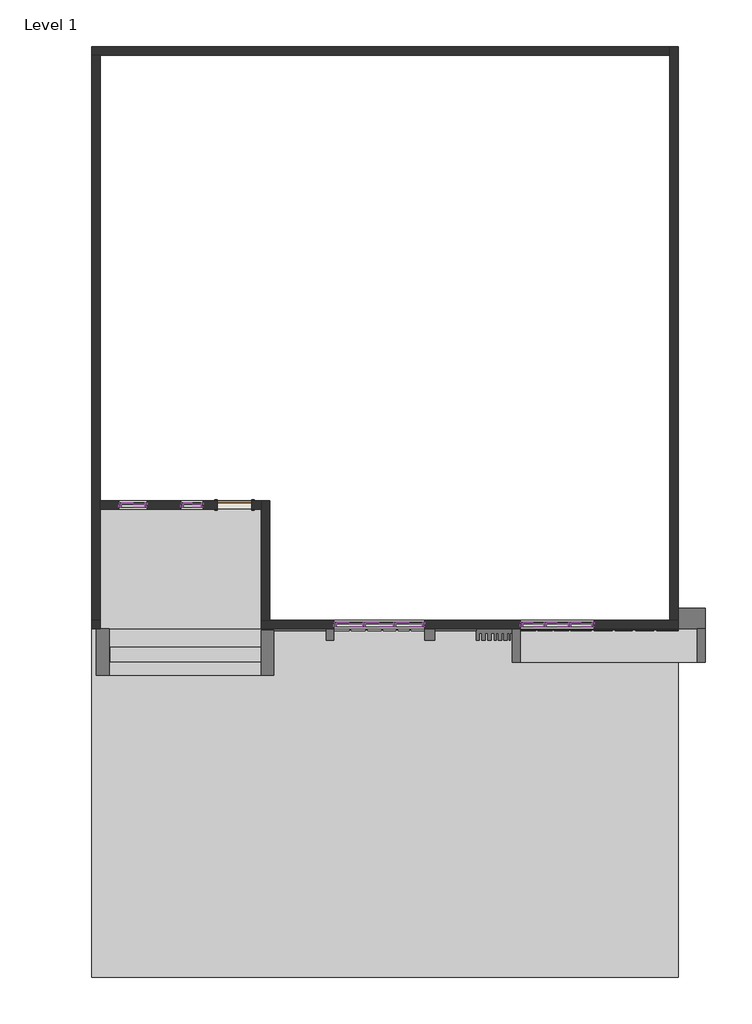
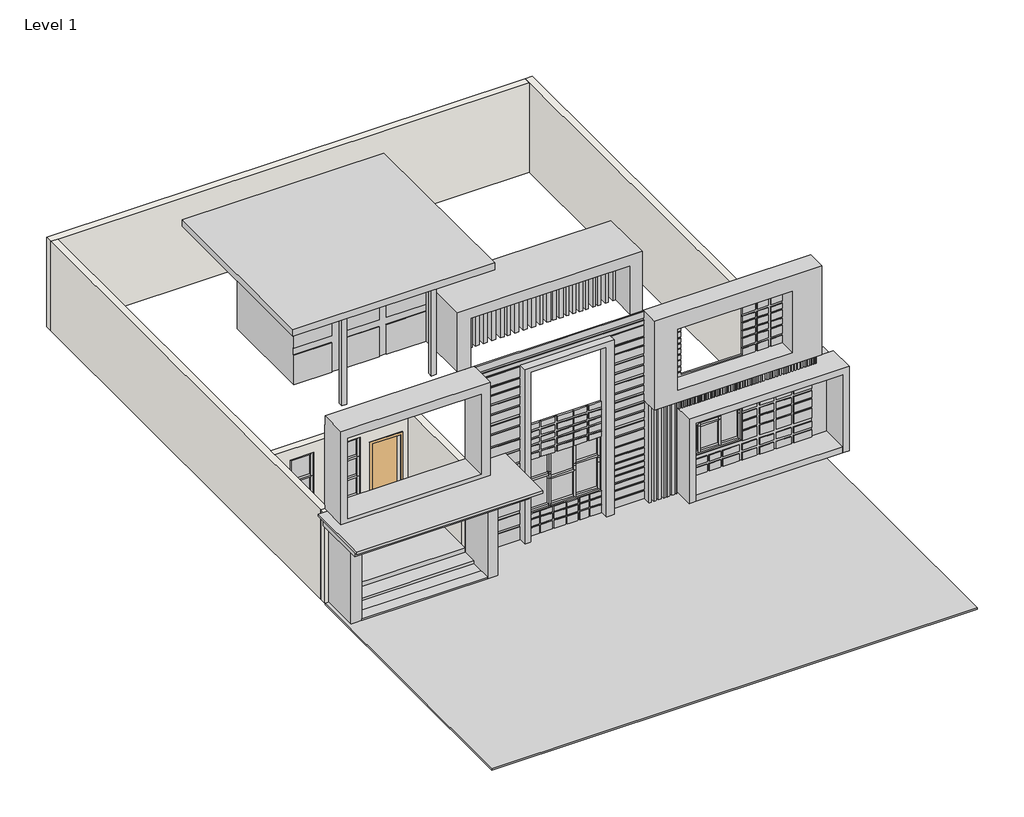
# One storey: 70 members, 18 plates, 7 walls, 4 proxies, 1 door.
"""IFC4 building model written with IfcOpenShell, lengths in millimetres."""

from ifc_helpers import new_model, si_unit, frame, origin, origin_with_axes, place, context, project, spatial, polyline, outline, extrude, faceted_brep, transform, mapped, element, save
from components import generic_models_1_generic_models_1_7cf849b9, generic_models_2_generic_models_2_6fa839af, generic_models_3_generic_models_3_82c5f115, generic_models_4_generic_models_4_69232215, generic_models_4_generic_models_4_6a6385c3, generic_models_4_generic_models_4_29f9d9a5, door_0ca8825f, member_3d7cb871, member_fb13da3b, member_6103f85b, member_00d00b53, member_cfc5edb3, member_86293703, member_cb167e66, member_a400357f, member_6f432376, member_8719ea0b, member_2af9f6c8, member_93756e10, member_876f8f00, member_abeaf8ac, member_f6f0dfdd, member_798d6cad, member_b689734a, member_9d02be77, member_7007ad49, member_b0b512a9, member_efb63d8e, member_802eba92, member_8b3492ed, member_01f21cfb, member_5e365d0c, member_12300432, member_86d06fe4, member_323df77c, member_1e736a25, system_panel_glazed_cdc3472a, system_panel_glazed_0523aacf, system_panel_glazed_d68d6f8b, system_panel_glazed_474a16cc, system_panel_glazed_52336633, system_panel_glazed_49caabb3, system_panel_glazed_917af8f4, system_panel_glazed_1be55c4b, system_panel_glazed_b40e79ec, system_panel_glazed_e688d5e8, system_panel_glazed_5707a053, system_panel_glazed_d7e326c9, system_panel_glazed_8c040c01, system_panel_glazed_3f46b533, system_panel_glazed_a9204d3a, system_panel_glazed_3a936e0b, system_panel_glazed_9f6ea25c

model = new_model("IFC4")

# Units and contexts
model_context = context("Model", 3, world=origin())
ifc_project = project(units=[si_unit("LENGTHUNIT", "METRE", prefix="MILLI")], contexts=[model_context])

# Site, building, storey
site = spatial("IfcSite", under=ifc_project)
building = spatial("IfcBuilding", under=site)
storey = spatial("IfcBuildingStorey", under=building, Name="Level 1", Elevation=0.0)

# Proxies
placement = place(None, origin())
generic_models_1_generic_models_1_shape = generic_models_1_generic_models_1_7cf849b9(model_context)
element("IfcBuildingElementProxy", 1, Name="Generic Models 1 : Generic Models 1", ObjectType="Generic Models 1 : Generic Models 1", at=placement, inside=storey, context=model_context, shape_type="MappedRepresentation", body=[
    mapped(generic_models_1_generic_models_1_shape, transform((0.0, 0.0, 0.0), x_axis=(1.0, 0.0, 0.0), y_axis=(0.0, 1.0, 0.0), z_axis=(0.0, 0.0, 1.0))),
])
generic_models_2_generic_models_2_shape = generic_models_2_generic_models_2_6fa839af(model_context)
element("IfcBuildingElementProxy", 2, Name="Generic Models 2 : Generic Models 2", ObjectType="Generic Models 2 : Generic Models 2", at=placement, inside=storey, context=model_context, shape_type="MappedRepresentation", body=[
    mapped(generic_models_2_generic_models_2_shape, transform((0.0, 0.0, 0.0), x_axis=(1.0, 0.0, 0.0), y_axis=(0.0, 1.0, 0.0), z_axis=(0.0, 0.0, 1.0))),
])
generic_models_3_generic_models_3_shape = generic_models_3_generic_models_3_82c5f115(model_context)
element("IfcBuildingElementProxy", 3, Name="Generic Models 3 : Generic Models 3", ObjectType="Generic Models 3 : Generic Models 3", at=placement, inside=storey, context=model_context, shape_type="MappedRepresentation", body=[
    mapped(generic_models_3_generic_models_3_shape, transform((0.0, 0.0, 0.0), x_axis=(1.0, 0.0, 0.0), y_axis=(0.0, 1.0, 0.0), z_axis=(0.0, 0.0, 1.0))),
])
generic_models_4_generic_models_4_shape = generic_models_4_generic_models_4_69232215(model_context)
generic_models_4_generic_models_4_2_shape = generic_models_4_generic_models_4_6a6385c3(model_context)
generic_models_4_generic_models_4_3_shape = generic_models_4_generic_models_4_29f9d9a5(model_context)
element("IfcBuildingElementProxy", 4, Name="Generic Models 4 : Generic Models 4", ObjectType="Generic Models 4 : Generic Models 4", at=placement, inside=storey, context=model_context, shape_type="MappedRepresentation", body=[
    mapped(generic_models_4_generic_models_4_shape, transform((0.0, 0.0, 0.0), x_axis=(1.0, 0.0, 0.0), y_axis=(0.0, 1.0, 0.0), z_axis=(0.0, 0.0, 1.0))),
    mapped(generic_models_4_generic_models_4_2_shape, transform((0.0, 0.0, 0.0), x_axis=(1.0, 0.0, 0.0), y_axis=(0.0, 1.0, 0.0), z_axis=(0.0, 0.0, 1.0))),
    mapped(generic_models_4_generic_models_4_3_shape, transform((0.0, 0.0, 0.0), x_axis=(1.0, 0.0, 0.0), y_axis=(0.0, 1.0, 0.0), z_axis=(0.0, 0.0, 1.0))),
])

# Door
door_shape = door_0ca8825f(model_context)
element("IfcDoor", 5, ObjectType="Single-Flush : 36\" x 84\"", at=placement, inside=storey, context=model_context, shape_type="MappedRepresentation", body=[
    mapped(door_shape, transform((-15502.789323, -10539.4538163, 203.2), x_axis=(1.0, 0.0, 0.0), y_axis=(0.0, 1.0, 0.0), z_axis=(0.0, 0.0, 1.0))),
])

# Members
member_shape = member_3d7cb871(model_context)
element("IfcMember", 6, ObjectType="Rectangular Mullion : 2.5\" x 5\" rectangular", at=placement, inside=storey, context=model_context, shape_type="MappedRepresentation", body=[
    mapped(member_shape, transform((-7854.214323, -13739.8538163, 1952.7546729), x_axis=(-1.0, 0.0, 0.0), y_axis=(0.0, -1.0, 0.0), z_axis=(0.0, 0.0, 1.0))),
])
element("IfcMember", 7, ObjectType="Rectangular Mullion : 2.5\" x 5\" rectangular", at=placement, inside=storey, context=model_context, shape_type="MappedRepresentation", body=[
    mapped(member_shape, transform((-12845.314323, -13739.8538163, 1907.2687583), x_axis=(-1.0, 0.0, 0.0), y_axis=(0.0, -1.0, 0.0), z_axis=(0.0, 0.0, 1.0))),
])
member_2_shape = member_fb13da3b(model_context)
element("IfcMember", 8, ObjectType="Rectangular Mullion : 2.5\" x 5\" rectangular", at=placement, inside=storey, context=model_context, shape_type="MappedRepresentation", body=[
    mapped(member_2_shape, transform((-7854.214323, -13739.8538163, 1876.5546729), x_axis=(-1.0, 0.0, 0.0), y_axis=(0.0, -1.0, 0.0), z_axis=(0.0, 0.0, 1.0))),
])
member_3_shape = member_6103f85b(model_context)
element("IfcMember", 9, ObjectType="Rectangular Mullion : 2.5\" x 5\" rectangular", at=placement, inside=storey, context=model_context, shape_type="MappedRepresentation", body=[
    mapped(member_3_shape, transform((-7225.564323, -13739.8538163, 1876.5546729), x_axis=(0.0, 0.0, 1.0), y_axis=(0.0, -1.0, 0.0), z_axis=(1.0, 0.0, 0.0))),
])
element("IfcMember", 10, ObjectType="Rectangular Mullion : 2.5\" x 5\" rectangular", at=placement, inside=storey, context=model_context, shape_type="MappedRepresentation", body=[
    mapped(member_3_shape, transform((-5936.514323, -13739.8538163, 1952.7546729), x_axis=(0.0, 0.0, 1.0), y_axis=(0.0, -1.0, 0.0), z_axis=(1.0, 0.0, 0.0))),
])
member_4_shape = member_00d00b53(model_context)
element("IfcMember", 11, ObjectType="Rectangular Mullion : 2.5\" x 5\" rectangular", at=placement, inside=storey, context=model_context, shape_type="MappedRepresentation", body=[
    mapped(member_4_shape, transform((-7193.814323, -13739.8538163, 1876.5546729), x_axis=(1.0, 0.0, 0.0), y_axis=(0.0, -1.0, 0.0), z_axis=(0.0, 0.0, -1.0))),
])
element("IfcMember", 12, ObjectType="Rectangular Mullion : 2.5\" x 5\" rectangular", at=placement, inside=storey, context=model_context, shape_type="MappedRepresentation", body=[
    mapped(member_4_shape, transform((-12032.514323, -13739.8538163, 1831.0687583), x_axis=(1.0, 0.0, 0.0), y_axis=(0.0, -1.0, 0.0), z_axis=(0.0, 0.0, -1.0))),
])
member_5_shape = member_cfc5edb3(model_context)
element("IfcMember", 13, ObjectType="Rectangular Mullion : 2.5\" x 5\" rectangular", at=placement, inside=storey, context=model_context, shape_type="MappedRepresentation", body=[
    mapped(member_5_shape, transform((-7193.814323, -13739.8538163, 1774.9546729), x_axis=(1.0, 0.0, 0.0), y_axis=(0.0, -1.0, 0.0), z_axis=(0.0, 0.0, -1.0))),
])
member_6_shape = member_86293703(model_context)
element("IfcMember", 14, ObjectType="Rectangular Mullion : 2.5\" x 5\" rectangular", at=placement, inside=storey, context=model_context, shape_type="MappedRepresentation", body=[
    mapped(member_6_shape, transform((-6565.164323, -13739.8538163, 1774.9546729), x_axis=(0.0, 0.0, 1.0), y_axis=(0.0, -1.0, 0.0), z_axis=(1.0, 0.0, 0.0))),
])
element("IfcMember", 15, ObjectType="Rectangular Mullion : 2.5\" x 5\" rectangular", at=placement, inside=storey, context=model_context, shape_type="MappedRepresentation", body=[
    mapped(member_5_shape, transform((-6533.414323, -13739.8538163, 1774.9546729), x_axis=(1.0, 0.0, 0.0), y_axis=(0.0, -1.0, 0.0), z_axis=(0.0, 0.0, -1.0))),
])
element("IfcMember", 16, ObjectType="Rectangular Mullion : 2.5\" x 5\" rectangular", at=placement, inside=storey, context=model_context, shape_type="MappedRepresentation", body=[
    mapped(member_4_shape, transform((-6533.414323, -13739.8538163, 1876.5546729), x_axis=(1.0, 0.0, 0.0), y_axis=(0.0, -1.0, 0.0), z_axis=(0.0, 0.0, -1.0))),
])
element("IfcMember", 17, ObjectType="Rectangular Mullion : 2.5\" x 5\" rectangular", at=placement, inside=storey, context=model_context, shape_type="MappedRepresentation", body=[
    mapped(member_4_shape, transform((-11219.714323, -13739.8538163, 1831.0687583), x_axis=(1.0, 0.0, 0.0), y_axis=(0.0, -1.0, 0.0), z_axis=(0.0, 0.0, -1.0))),
])
member_7_shape = member_cb167e66(model_context)
element("IfcMember", 18, ObjectType="Rectangular Mullion : 2.5\" x 5\" rectangular", at=placement, inside=storey, context=model_context, shape_type="MappedRepresentation", body=[
    mapped(member_7_shape, transform((-7193.814323, -13739.8538163, 872.4244956), x_axis=(1.0, 0.0, 0.0), y_axis=(0.0, -1.0, 0.0), z_axis=(0.0, 0.0, -1.0))),
])
element("IfcMember", 19, ObjectType="Rectangular Mullion : 2.5\" x 5\" rectangular", at=placement, inside=storey, context=model_context, shape_type="MappedRepresentation", body=[
    mapped(member_7_shape, transform((-6533.414323, -13739.8538163, 872.4244956), x_axis=(1.0, 0.0, 0.0), y_axis=(0.0, -1.0, 0.0), z_axis=(0.0, 0.0, -1.0))),
])
member_8_shape = member_a400357f(model_context)
element("IfcMember", 20, ObjectType="Rectangular Mullion : 2.5\" x 5\" rectangular", at=placement, inside=storey, context=model_context, shape_type="MappedRepresentation", body=[
    mapped(member_8_shape, transform((-7162.064323, -13739.8538163, 872.4244956), x_axis=(0.0, 0.0, -1.0), y_axis=(0.0, -1.0, 0.0), z_axis=(-1.0, 0.0, 0.0))),
])
member_9_shape = member_6f432376(model_context)
element("IfcMember", 21, ObjectType="Rectangular Mullion : 2.5\" x 5\" rectangular", at=placement, inside=storey, context=model_context, shape_type="MappedRepresentation", body=[
    mapped(member_9_shape, transform((-6501.664323, -13739.8538163, 872.4244956), x_axis=(0.0, 0.0, -1.0), y_axis=(0.0, -1.0, 0.0), z_axis=(-1.0, 0.0, 0.0))),
])
element("IfcMember", 22, ObjectType="Rectangular Mullion : 2.5\" x 5\" rectangular", at=placement, inside=storey, context=model_context, shape_type="MappedRepresentation", body=[
    mapped(member_9_shape, transform((-7790.714323, -13739.8538163, 872.4244956), x_axis=(0.0, 0.0, -1.0), y_axis=(0.0, -1.0, 0.0), z_axis=(-1.0, 0.0, 0.0))),
])
member_10_shape = member_8719ea0b(model_context)
element("IfcMember", 23, ObjectType="Rectangular Mullion : 2.5\" x 5\" rectangular", at=placement, inside=storey, context=model_context, shape_type="MappedRepresentation", body=[
    mapped(member_10_shape, transform((-7854.214323, -13739.8538163, 1774.9546729), x_axis=(-1.0, 0.0, 0.0), y_axis=(0.0, -1.0, 0.0), z_axis=(0.0, 0.0, 1.0))),
])
member_11_shape = member_2af9f6c8(model_context)
element("IfcMember", 24, ObjectType="Rectangular Mullion : 2.5\" x 5\" rectangular", at=placement, inside=storey, context=model_context, shape_type="MappedRepresentation", body=[
    mapped(member_11_shape, transform((-7193.814323, -13739.8538163, 1952.7546729), x_axis=(1.0, 0.0, 0.0), y_axis=(0.0, -1.0, 0.0), z_axis=(0.0, 0.0, -1.0))),
])
element("IfcMember", 25, ObjectType="Rectangular Mullion : 2.5\" x 5\" rectangular", at=placement, inside=storey, context=model_context, shape_type="MappedRepresentation", body=[
    mapped(member_11_shape, transform((-6533.414323, -13739.8538163, 1952.7546729), x_axis=(1.0, 0.0, 0.0), y_axis=(0.0, -1.0, 0.0), z_axis=(0.0, 0.0, -1.0))),
])
element("IfcMember", 26, ObjectType="Rectangular Mullion : 2.5\" x 5\" rectangular", at=placement, inside=storey, context=model_context, shape_type="MappedRepresentation", body=[
    mapped(member_9_shape, transform((-7225.564323, -13739.8538163, 2677.4848502), x_axis=(0.0, 0.0, 1.0), y_axis=(0.0, -1.0, 0.0), z_axis=(1.0, 0.0, 0.0))),
])
element("IfcMember", 27, ObjectType="Rectangular Mullion : 2.5\" x 5\" rectangular", at=placement, inside=storey, context=model_context, shape_type="MappedRepresentation", body=[
    mapped(member_9_shape, transform((-5936.514323, -13739.8538163, 2677.4848502), x_axis=(0.0, 0.0, 1.0), y_axis=(0.0, -1.0, 0.0), z_axis=(1.0, 0.0, 0.0))),
])
element("IfcMember", 28, ObjectType="Rectangular Mullion : 2.5\" x 5\" rectangular", at=placement, inside=storey, context=model_context, shape_type="MappedRepresentation", body=[
    mapped(member_8_shape, transform((-6565.164323, -13739.8538163, 2677.4848502), x_axis=(0.0, 0.0, 1.0), y_axis=(0.0, -1.0, 0.0), z_axis=(1.0, 0.0, 0.0))),
])
member_12_shape = member_93756e10(model_context)
element("IfcMember", 29, ObjectType="Rectangular Mullion : 2.5\" x 5\" rectangular", at=placement, inside=storey, context=model_context, shape_type="MappedRepresentation", body=[
    mapped(member_12_shape, transform((-7854.214323, -13739.8538163, 2677.4848502), x_axis=(-1.0, 0.0, 0.0), y_axis=(0.0, -1.0, 0.0), z_axis=(0.0, 0.0, 1.0))),
])
member_13_shape = member_876f8f00(model_context)
element("IfcMember", 30, ObjectType="Rectangular Mullion : 2.5\" x 5\" rectangular", at=placement, inside=storey, context=model_context, shape_type="MappedRepresentation", body=[
    mapped(member_13_shape, transform((-12845.314323, -13739.8538163, 1831.0687583), x_axis=(-1.0, 0.0, 0.0), y_axis=(0.0, -1.0, 0.0), z_axis=(0.0, 0.0, 1.0))),
])
member_14_shape = member_abeaf8ac(model_context)
element("IfcMember", 31, ObjectType="Rectangular Mullion : 2.5\" x 5\" rectangular", at=placement, inside=storey, context=model_context, shape_type="MappedRepresentation", body=[
    mapped(member_14_shape, transform((-12064.264323, -13739.8538163, 1831.0687583), x_axis=(0.0, 0.0, 1.0), y_axis=(0.0, -1.0, 0.0), z_axis=(1.0, 0.0, 0.0))),
])
element("IfcMember", 32, ObjectType="Rectangular Mullion : 2.5\" x 5\" rectangular", at=placement, inside=storey, context=model_context, shape_type="MappedRepresentation", body=[
    mapped(member_14_shape, transform((-10470.414323, -13739.8538163, 1907.2687583), x_axis=(0.0, 0.0, 1.0), y_axis=(0.0, -1.0, 0.0), z_axis=(1.0, 0.0, 0.0))),
])
member_15_shape = member_f6f0dfdd(model_context)
element("IfcMember", 33, ObjectType="Rectangular Mullion : 2.5\" x 5\" rectangular", at=placement, inside=storey, context=model_context, shape_type="MappedRepresentation", body=[
    mapped(member_15_shape, transform((-12032.514323, -13739.8538163, 1678.6687583), x_axis=(1.0, 0.0, 0.0), y_axis=(0.0, -1.0, 0.0), z_axis=(0.0, 0.0, -1.0))),
])
member_16_shape = member_798d6cad(model_context)
element("IfcMember", 34, ObjectType="Rectangular Mullion : 2.5\" x 5\" rectangular", at=placement, inside=storey, context=model_context, shape_type="MappedRepresentation", body=[
    mapped(member_16_shape, transform((-11251.464323, -13739.8538163, 1678.6687583), x_axis=(0.0, 0.0, 1.0), y_axis=(0.0, -1.0, 0.0), z_axis=(1.0, 0.0, 0.0))),
])
element("IfcMember", 35, ObjectType="Rectangular Mullion : 2.5\" x 5\" rectangular", at=placement, inside=storey, context=model_context, shape_type="MappedRepresentation", body=[
    mapped(member_15_shape, transform((-11219.714323, -13739.8538163, 1678.6687583), x_axis=(1.0, 0.0, 0.0), y_axis=(0.0, -1.0, 0.0), z_axis=(0.0, 0.0, -1.0))),
])
member_17_shape = member_b689734a(model_context)
element("IfcMember", 36, ObjectType="Rectangular Mullion : 2.5\" x 5\" rectangular", at=placement, inside=storey, context=model_context, shape_type="MappedRepresentation", body=[
    mapped(member_17_shape, transform((-12032.514323, -13739.8538163, 753.9093053), x_axis=(1.0, 0.0, 0.0), y_axis=(0.0, -1.0, 0.0), z_axis=(0.0, 0.0, -1.0))),
])
element("IfcMember", 37, ObjectType="Rectangular Mullion : 2.5\" x 5\" rectangular", at=placement, inside=storey, context=model_context, shape_type="MappedRepresentation", body=[
    mapped(member_17_shape, transform((-11219.714323, -13739.8538163, 753.9093053), x_axis=(1.0, 0.0, 0.0), y_axis=(0.0, -1.0, 0.0), z_axis=(0.0, 0.0, -1.0))),
])
member_18_shape = member_9d02be77(model_context)
element("IfcMember", 38, ObjectType="Rectangular Mullion : 2.5\" x 5\" rectangular", at=placement, inside=storey, context=model_context, shape_type="MappedRepresentation", body=[
    mapped(member_18_shape, transform((-12000.764323, -13739.8538163, 753.9093053), x_axis=(0.0, 0.0, -1.0), y_axis=(0.0, -1.0, 0.0), z_axis=(-1.0, 0.0, 0.0))),
])
member_19_shape = member_7007ad49(model_context)
element("IfcMember", 39, ObjectType="Rectangular Mullion : 2.5\" x 5\" rectangular", at=placement, inside=storey, context=model_context, shape_type="MappedRepresentation", body=[
    mapped(member_19_shape, transform((-11187.964323, -13739.8538163, 753.9093053), x_axis=(0.0, 0.0, -1.0), y_axis=(0.0, -1.0, 0.0), z_axis=(-1.0, 0.0, 0.0))),
])
element("IfcMember", 40, ObjectType="Rectangular Mullion : 2.5\" x 5\" rectangular", at=placement, inside=storey, context=model_context, shape_type="MappedRepresentation", body=[
    mapped(member_19_shape, transform((-12781.814323, -13739.8538163, 753.9093053), x_axis=(0.0, 0.0, -1.0), y_axis=(0.0, -1.0, 0.0), z_axis=(-1.0, 0.0, 0.0))),
])
member_20_shape = member_b0b512a9(model_context)
element("IfcMember", 41, ObjectType="Rectangular Mullion : 2.5\" x 5\" rectangular", at=placement, inside=storey, context=model_context, shape_type="MappedRepresentation", body=[
    mapped(member_20_shape, transform((-12845.314323, -13739.8538163, 1678.6687583), x_axis=(-1.0, 0.0, 0.0), y_axis=(0.0, -1.0, 0.0), z_axis=(0.0, 0.0, 1.0))),
])
element("IfcMember", 42, ObjectType="Rectangular Mullion : 2.5\" x 5\" rectangular", at=placement, inside=storey, context=model_context, shape_type="MappedRepresentation", body=[
    mapped(member_shape, transform((-10406.914323, -13739.8538163, 1831.0687583), x_axis=(1.0, 0.0, 0.0), y_axis=(0.0, -1.0, 0.0), z_axis=(0.0, 0.0, -1.0))),
])
element("IfcMember", 43, ObjectType="Rectangular Mullion : 2.5\" x 5\" rectangular", at=placement, inside=storey, context=model_context, shape_type="MappedRepresentation", body=[
    mapped(member_shape, transform((-5873.014323, -13739.8538163, 1876.5546729), x_axis=(1.0, 0.0, 0.0), y_axis=(0.0, -1.0, 0.0), z_axis=(0.0, 0.0, -1.0))),
])
element("IfcMember", 44, ObjectType="Rectangular Mullion : 2.5\" x 5\" rectangular", at=placement, inside=storey, context=model_context, shape_type="MappedRepresentation", body=[
    mapped(member_13_shape, transform((-10406.914323, -13739.8538163, 1678.6687583), x_axis=(1.0, 0.0, 0.0), y_axis=(0.0, -1.0, 0.0), z_axis=(0.0, 0.0, -1.0))),
])
element("IfcMember", 45, ObjectType="Rectangular Mullion : 2.5\" x 5\" rectangular", at=placement, inside=storey, context=model_context, shape_type="MappedRepresentation", body=[
    mapped(member_20_shape, transform((-10406.914323, -13739.8538163, 753.9093053), x_axis=(1.0, 0.0, 0.0), y_axis=(0.0, -1.0, 0.0), z_axis=(0.0, 0.0, -1.0))),
])
member_21_shape = member_efb63d8e(model_context)
element("IfcMember", 46, ObjectType="Rectangular Mullion : 2.5\" x 5\" rectangular", at=placement, inside=storey, context=model_context, shape_type="MappedRepresentation", body=[
    mapped(member_21_shape, transform((-12032.514323, -13739.8538163, 1907.2687583), x_axis=(1.0, 0.0, 0.0), y_axis=(0.0, -1.0, 0.0), z_axis=(0.0, 0.0, -1.0))),
])
element("IfcMember", 47, ObjectType="Rectangular Mullion : 2.5\" x 5\" rectangular", at=placement, inside=storey, context=model_context, shape_type="MappedRepresentation", body=[
    mapped(member_21_shape, transform((-11219.714323, -13739.8538163, 1907.2687583), x_axis=(1.0, 0.0, 0.0), y_axis=(0.0, -1.0, 0.0), z_axis=(0.0, 0.0, -1.0))),
])
element("IfcMember", 48, ObjectType="Rectangular Mullion : 2.5\" x 5\" rectangular", at=placement, inside=storey, context=model_context, shape_type="MappedRepresentation", body=[
    mapped(member_18_shape, transform((-11251.464323, -13739.8538163, 2603.4282114), x_axis=(0.0, 0.0, 1.0), y_axis=(0.0, -1.0, 0.0), z_axis=(1.0, 0.0, 0.0))),
])
element("IfcMember", 49, ObjectType="Rectangular Mullion : 2.5\" x 5\" rectangular", at=placement, inside=storey, context=model_context, shape_type="MappedRepresentation", body=[
    mapped(member_19_shape, transform((-12064.264323, -13739.8538163, 2603.4282114), x_axis=(0.0, 0.0, 1.0), y_axis=(0.0, -1.0, 0.0), z_axis=(1.0, 0.0, 0.0))),
])
element("IfcMember", 50, ObjectType="Rectangular Mullion : 2.5\" x 5\" rectangular", at=placement, inside=storey, context=model_context, shape_type="MappedRepresentation", body=[
    mapped(member_19_shape, transform((-10470.414323, -13739.8538163, 2603.4282114), x_axis=(0.0, 0.0, 1.0), y_axis=(0.0, -1.0, 0.0), z_axis=(1.0, 0.0, 0.0))),
])
member_22_shape = member_802eba92(model_context)
element("IfcMember", 51, ObjectType="Rectangular Mullion : 2.5\" x 5\" rectangular", at=placement, inside=storey, context=model_context, shape_type="MappedRepresentation", body=[
    mapped(member_22_shape, transform((-12845.314323, -13739.8538163, 2603.4282114), x_axis=(-1.0, 0.0, 0.0), y_axis=(0.0, -1.0, 0.0), z_axis=(0.0, 0.0, 1.0))),
])
element("IfcMember", 52, ObjectType="Rectangular Mullion : 2.5\" x 5\" rectangular", at=placement, inside=storey, context=model_context, shape_type="MappedRepresentation", body=[
    mapped(member_22_shape, transform((-10406.914323, -13739.8538163, 1907.2687583), x_axis=(1.0, 0.0, 0.0), y_axis=(0.0, -1.0, 0.0), z_axis=(0.0, 0.0, -1.0))),
])
member_23_shape = member_8b3492ed(model_context)
element("IfcMember", 53, ObjectType="Rectangular Mullion : 2.5\" x 5\" rectangular", at=placement, inside=storey, context=model_context, shape_type="MappedRepresentation", body=[
    mapped(member_23_shape, transform((-18598.414323, -10539.4538163, 2686.6585234), x_axis=(-1.0, 0.0, 0.0), y_axis=(0.0, -1.0, 0.0), z_axis=(0.0, 0.0, 1.0))),
])
member_24_shape = member_01f21cfb(model_context)
element("IfcMember", 54, ObjectType="Rectangular Mullion : 2.5\" x 5\" rectangular", at=placement, inside=storey, context=model_context, shape_type="MappedRepresentation", body=[
    mapped(member_24_shape, transform((-18598.414323, -10539.4538163, 1873.8585234), x_axis=(-1.0, 0.0, 0.0), y_axis=(0.0, -1.0, 0.0), z_axis=(0.0, 0.0, 1.0))),
])
element("IfcMember", 55, ObjectType="Rectangular Mullion : 2.5\" x 5\" rectangular", at=placement, inside=storey, context=model_context, shape_type="MappedRepresentation", body=[
    mapped(member_24_shape, transform((-18598.414323, -10539.4538163, 1256.6236446), x_axis=(-1.0, 0.0, 0.0), y_axis=(0.0, -1.0, 0.0), z_axis=(0.0, 0.0, 1.0))),
])
member_25_shape = member_5e365d0c(model_context)
element("IfcMember", 56, ObjectType="Rectangular Mullion : 2.5\" x 5\" rectangular", at=placement, inside=storey, context=model_context, shape_type="MappedRepresentation", body=[
    mapped(member_25_shape, transform((-17899.914323, -10539.4538163, 2686.6585234), x_axis=(0.0, 0.0, 1.0), y_axis=(0.0, -1.0, 0.0), z_axis=(1.0, 0.0, 0.0))),
])
member_26_shape = member_12300432(model_context)
element("IfcMember", 57, ObjectType="Rectangular Mullion : 2.5\" x 5\" rectangular", at=placement, inside=storey, context=model_context, shape_type="MappedRepresentation", body=[
    mapped(member_26_shape, transform((-17899.914323, -10539.4538163, 1873.8585234), x_axis=(0.0, 0.0, 1.0), y_axis=(0.0, -1.0, 0.0), z_axis=(1.0, 0.0, 0.0))),
])
element("IfcMember", 58, ObjectType="Rectangular Mullion : 2.5\" x 5\" rectangular", at=placement, inside=storey, context=model_context, shape_type="MappedRepresentation", body=[
    mapped(member_26_shape, transform((-17899.914323, -10539.4538163, 1256.6236446), x_axis=(0.0, 0.0, 1.0), y_axis=(0.0, -1.0, 0.0), z_axis=(1.0, 0.0, 0.0))),
])
element("IfcMember", 59, ObjectType="Rectangular Mullion : 2.5\" x 5\" rectangular", at=placement, inside=storey, context=model_context, shape_type="MappedRepresentation", body=[
    mapped(member_25_shape, transform((-18534.914323, -10539.4538163, 639.3887658), x_axis=(0.0, 0.0, -1.0), y_axis=(0.0, -1.0, 0.0), z_axis=(-1.0, 0.0, 0.0))),
])
element("IfcMember", 60, ObjectType="Rectangular Mullion : 2.5\" x 5\" rectangular", at=placement, inside=storey, context=model_context, shape_type="MappedRepresentation", body=[
    mapped(member_24_shape, transform((-17836.414323, -10539.4538163, 1256.6236446), x_axis=(1.0, 0.0, 0.0), y_axis=(0.0, -1.0, 0.0), z_axis=(0.0, 0.0, -1.0))),
])
element("IfcMember", 61, ObjectType="Rectangular Mullion : 2.5\" x 5\" rectangular", at=placement, inside=storey, context=model_context, shape_type="MappedRepresentation", body=[
    mapped(member_23_shape, transform((-17836.414323, -10539.4538163, 1873.8585234), x_axis=(1.0, 0.0, 0.0), y_axis=(0.0, -1.0, 0.0), z_axis=(0.0, 0.0, -1.0))),
])
element("IfcMember", 62, ObjectType="Rectangular Mullion : 2.5\" x 5\" rectangular", at=placement, inside=storey, context=model_context, shape_type="MappedRepresentation", body=[
    mapped(member_24_shape, transform((-17836.414323, -10539.4538163, 639.3887658), x_axis=(1.0, 0.0, 0.0), y_axis=(0.0, -1.0, 0.0), z_axis=(0.0, 0.0, -1.0))),
])
member_27_shape = member_86d06fe4(model_context)
element("IfcMember", 63, ObjectType="Rectangular Mullion : 2.5\" x 5\" rectangular", at=placement, inside=storey, context=model_context, shape_type="MappedRepresentation", body=[
    mapped(member_27_shape, transform((-16394.964323, -10539.4538163, 2678.7342332), x_axis=(0.0, 0.0, 1.0), y_axis=(0.0, -1.0, 0.0), z_axis=(1.0, 0.0, 0.0))),
])
member_28_shape = member_323df77c(model_context)
element("IfcMember", 64, ObjectType="Rectangular Mullion : 2.5\" x 5\" rectangular", at=placement, inside=storey, context=model_context, shape_type="MappedRepresentation", body=[
    mapped(member_28_shape, transform((-16394.964323, -10539.4538163, 2006.619489), x_axis=(0.0, 0.0, 1.0), y_axis=(0.0, -1.0, 0.0), z_axis=(1.0, 0.0, 0.0))),
])
element("IfcMember", 65, ObjectType="Rectangular Mullion : 2.5\" x 5\" rectangular", at=placement, inside=storey, context=model_context, shape_type="MappedRepresentation", body=[
    mapped(member_28_shape, transform((-16394.964323, -10539.4538163, 1334.5047448), x_axis=(0.0, 0.0, 1.0), y_axis=(0.0, -1.0, 0.0), z_axis=(1.0, 0.0, 0.0))),
])
member_29_shape = member_1e736a25(model_context)
element("IfcMember", 66, ObjectType="Rectangular Mullion : 2.5\" x 5\" rectangular", at=placement, inside=storey, context=model_context, shape_type="MappedRepresentation", body=[
    mapped(member_29_shape, transform((-16941.064323, -10539.4538163, 2678.7342332), x_axis=(-1.0, 0.0, 0.0), y_axis=(0.0, -1.0, 0.0), z_axis=(0.0, 0.0, 1.0))),
])
element("IfcMember", 67, ObjectType="Rectangular Mullion : 2.5\" x 5\" rectangular", at=placement, inside=storey, context=model_context, shape_type="MappedRepresentation", body=[
    mapped(member_29_shape, transform((-16331.464323, -10539.4538163, 2006.619489), x_axis=(1.0, 0.0, 0.0), y_axis=(0.0, -1.0, 0.0), z_axis=(0.0, 0.0, -1.0))),
])
element("IfcMember", 68, ObjectType="Rectangular Mullion : 2.5\" x 5\" rectangular", at=placement, inside=storey, context=model_context, shape_type="MappedRepresentation", body=[
    mapped(member_29_shape, transform((-16941.064323, -10539.4538163, 2006.619489), x_axis=(-1.0, 0.0, 0.0), y_axis=(0.0, -1.0, 0.0), z_axis=(0.0, 0.0, 1.0))),
])
element("IfcMember", 69, ObjectType="Rectangular Mullion : 2.5\" x 5\" rectangular", at=placement, inside=storey, context=model_context, shape_type="MappedRepresentation", body=[
    mapped(member_29_shape, transform((-16331.464323, -10539.4538163, 1334.5047448), x_axis=(1.0, 0.0, 0.0), y_axis=(0.0, -1.0, 0.0), z_axis=(0.0, 0.0, -1.0))),
])
element("IfcMember", 70, ObjectType="Rectangular Mullion : 2.5\" x 5\" rectangular", at=placement, inside=storey, context=model_context, shape_type="MappedRepresentation", body=[
    mapped(member_27_shape, transform((-16877.564323, -10539.4538163, 662.3900006), x_axis=(0.0, 0.0, -1.0), y_axis=(0.0, -1.0, 0.0), z_axis=(-1.0, 0.0, 0.0))),
])
element("IfcMember", 71, ObjectType="Rectangular Mullion : 2.5\" x 5\" rectangular", at=placement, inside=storey, context=model_context, shape_type="MappedRepresentation", body=[
    mapped(member_29_shape, transform((-16941.064323, -10539.4538163, 1334.5047448), x_axis=(-1.0, 0.0, 0.0), y_axis=(0.0, -1.0, 0.0), z_axis=(0.0, 0.0, 1.0))),
])
element("IfcMember", 72, ObjectType="Rectangular Mullion : 2.5\" x 5\" rectangular", at=placement, inside=storey, context=model_context, shape_type="MappedRepresentation", body=[
    mapped(member_29_shape, transform((-16331.464323, -10539.4538163, 662.3900006), x_axis=(1.0, 0.0, 0.0), y_axis=(0.0, -1.0, 0.0), z_axis=(0.0, 0.0, -1.0))),
])
element("IfcMember", 73, ObjectType="Rectangular Mullion : 2.5\" x 5\" rectangular", at=placement, inside=storey, context=model_context, shape_type="MappedRepresentation", body=[
    mapped(member_12_shape, transform((-5873.014323, -13739.8538163, 1952.7546729), x_axis=(1.0, 0.0, 0.0), y_axis=(0.0, -1.0, 0.0), z_axis=(0.0, 0.0, -1.0))),
])
element("IfcMember", 74, ObjectType="Rectangular Mullion : 2.5\" x 5\" rectangular", at=placement, inside=storey, context=model_context, shape_type="MappedRepresentation", body=[
    mapped(member_2_shape, transform((-5873.014323, -13739.8538163, 1774.9546729), x_axis=(1.0, 0.0, 0.0), y_axis=(0.0, -1.0, 0.0), z_axis=(0.0, 0.0, -1.0))),
])
element("IfcMember", 75, ObjectType="Rectangular Mullion : 2.5\" x 5\" rectangular", at=placement, inside=storey, context=model_context, shape_type="MappedRepresentation", body=[
    mapped(member_10_shape, transform((-5873.014323, -13739.8538163, 872.4244956), x_axis=(1.0, 0.0, 0.0), y_axis=(0.0, -1.0, 0.0), z_axis=(0.0, 0.0, -1.0))),
])

# Plates
system_panel_glazed_shape = system_panel_glazed_cdc3472a(model_context)
element("IfcPlate", 76, ObjectType="System Panel : Glazed", at=placement, inside=storey, context=model_context, shape_type="MappedRepresentation", body=[
    mapped(system_panel_glazed_shape, transform((-7508.139323, -13739.8538163, 935.9244956), x_axis=(1.0, 0.0, 0.0), y_axis=(0.0, 1.0, 0.0), z_axis=(0.0, 0.0, 1.0))),
])
system_panel_glazed_2_shape = system_panel_glazed_0523aacf(model_context)
element("IfcPlate", 77, ObjectType="System Panel : Glazed", at=placement, inside=storey, context=model_context, shape_type="MappedRepresentation", body=[
    mapped(system_panel_glazed_2_shape, transform((-6863.614323, -13739.8538163, 935.9244956), x_axis=(1.0, 0.0, 0.0), y_axis=(0.0, 1.0, 0.0), z_axis=(0.0, 0.0, 1.0))),
])
system_panel_glazed_3_shape = system_panel_glazed_d68d6f8b(model_context)
element("IfcPlate", 78, ObjectType="System Panel : Glazed", at=placement, inside=storey, context=model_context, shape_type="MappedRepresentation", body=[
    mapped(system_panel_glazed_3_shape, transform((-6863.614323, -13739.8538163, 1806.7046729), x_axis=(1.0, 0.0, 0.0), y_axis=(0.0, 1.0, 0.0), z_axis=(0.0, 0.0, 1.0))),
])
system_panel_glazed_4_shape = system_panel_glazed_474a16cc(model_context)
element("IfcPlate", 79, ObjectType="System Panel : Glazed", at=placement, inside=storey, context=model_context, shape_type="MappedRepresentation", body=[
    mapped(system_panel_glazed_4_shape, transform((-7508.139323, -13739.8538163, 1908.3046729), x_axis=(1.0, 0.0, 0.0), y_axis=(0.0, 1.0, 0.0), z_axis=(0.0, 0.0, 1.0))),
])
system_panel_glazed_5_shape = system_panel_glazed_52336633(model_context)
element("IfcPlate", 80, ObjectType="System Panel : Glazed", at=placement, inside=storey, context=model_context, shape_type="MappedRepresentation", body=[
    mapped(system_panel_glazed_5_shape, transform((-12423.039323, -13739.8538163, 817.4093053), x_axis=(1.0, 0.0, 0.0), y_axis=(0.0, 1.0, 0.0), z_axis=(0.0, 0.0, 1.0))),
])
system_panel_glazed_6_shape = system_panel_glazed_49caabb3(model_context)
element("IfcPlate", 81, ObjectType="System Panel : Glazed", at=placement, inside=storey, context=model_context, shape_type="MappedRepresentation", body=[
    mapped(system_panel_glazed_6_shape, transform((-11626.114323, -13739.8538163, 817.4093053), x_axis=(1.0, 0.0, 0.0), y_axis=(0.0, 1.0, 0.0), z_axis=(0.0, 0.0, 1.0))),
])
system_panel_glazed_7_shape = system_panel_glazed_917af8f4(model_context)
element("IfcPlate", 82, ObjectType="System Panel : Glazed", at=placement, inside=storey, context=model_context, shape_type="MappedRepresentation", body=[
    mapped(system_panel_glazed_7_shape, transform((-10829.189323, -13739.8538163, 817.4093053), x_axis=(1.0, 0.0, 0.0), y_axis=(0.0, 1.0, 0.0), z_axis=(0.0, 0.0, 1.0))),
])
system_panel_glazed_8_shape = system_panel_glazed_1be55c4b(model_context)
element("IfcPlate", 83, ObjectType="System Panel : Glazed", at=placement, inside=storey, context=model_context, shape_type="MappedRepresentation", body=[
    mapped(system_panel_glazed_8_shape, transform((-11626.114323, -13739.8538163, 1710.4187583), x_axis=(1.0, 0.0, 0.0), y_axis=(0.0, 1.0, 0.0), z_axis=(0.0, 0.0, 1.0))),
])
system_panel_glazed_9_shape = system_panel_glazed_b40e79ec(model_context)
element("IfcPlate", 84, ObjectType="System Panel : Glazed", at=placement, inside=storey, context=model_context, shape_type="MappedRepresentation", body=[
    mapped(system_panel_glazed_9_shape, transform((-12423.039323, -13739.8538163, 1862.8187583), x_axis=(1.0, 0.0, 0.0), y_axis=(0.0, 1.0, 0.0), z_axis=(0.0, 0.0, 1.0))),
])
system_panel_glazed_10_shape = system_panel_glazed_e688d5e8(model_context)
element("IfcPlate", 85, ObjectType="System Panel : Glazed", at=placement, inside=storey, context=model_context, shape_type="MappedRepresentation", body=[
    mapped(system_panel_glazed_10_shape, transform((-10829.189323, -13739.8538163, 1939.0187583), x_axis=(1.0, 0.0, 0.0), y_axis=(0.0, 1.0, 0.0), z_axis=(0.0, 0.0, 1.0))),
])
system_panel_glazed_11_shape = system_panel_glazed_5707a053(model_context)
element("IfcPlate", 86, ObjectType="System Panel : Glazed", at=placement, inside=storey, context=model_context, shape_type="MappedRepresentation", body=[
    mapped(system_panel_glazed_11_shape, transform((-18217.414323, -10539.4538163, 702.8887658), x_axis=(1.0, 0.0, 0.0), y_axis=(0.0, 1.0, 0.0), z_axis=(0.0, 0.0, 1.0))),
])
system_panel_glazed_12_shape = system_panel_glazed_d7e326c9(model_context)
element("IfcPlate", 87, ObjectType="System Panel : Glazed", at=placement, inside=storey, context=model_context, shape_type="MappedRepresentation", body=[
    mapped(system_panel_glazed_12_shape, transform((-18217.414323, -10539.4538163, 1905.6085234), x_axis=(1.0, 0.0, 0.0), y_axis=(0.0, 1.0, 0.0), z_axis=(0.0, 0.0, 1.0))),
])
system_panel_glazed_13_shape = system_panel_glazed_8c040c01(model_context)
element("IfcPlate", 88, ObjectType="System Panel : Glazed", at=placement, inside=storey, context=model_context, shape_type="MappedRepresentation", body=[
    mapped(system_panel_glazed_13_shape, transform((-18217.414323, -10539.4538163, 1288.3736446), x_axis=(1.0, 0.0, 0.0), y_axis=(0.0, 1.0, 0.0), z_axis=(0.0, 0.0, 1.0))),
])
system_panel_glazed_14_shape = system_panel_glazed_3f46b533(model_context)
element("IfcPlate", 89, ObjectType="System Panel : Glazed", at=placement, inside=storey, context=model_context, shape_type="MappedRepresentation", body=[
    mapped(system_panel_glazed_14_shape, transform((-16636.264323, -10539.4538163, 725.8900006), x_axis=(1.0, 0.0, 0.0), y_axis=(0.0, 1.0, 0.0), z_axis=(0.0, 0.0, 1.0))),
])
element("IfcPlate", 90, ObjectType="System Panel : Glazed", at=placement, inside=storey, context=model_context, shape_type="MappedRepresentation", body=[
    mapped(system_panel_glazed_14_shape, transform((-16636.264323, -10539.4538163, 2038.369489), x_axis=(1.0, 0.0, 0.0), y_axis=(0.0, 1.0, 0.0), z_axis=(0.0, 0.0, 1.0))),
])
system_panel_glazed_15_shape = system_panel_glazed_a9204d3a(model_context)
element("IfcPlate", 91, ObjectType="System Panel : Glazed", at=placement, inside=storey, context=model_context, shape_type="MappedRepresentation", body=[
    mapped(system_panel_glazed_15_shape, transform((-16636.264323, -10539.4538163, 1366.2547448), x_axis=(1.0, 0.0, 0.0), y_axis=(0.0, 1.0, 0.0), z_axis=(0.0, 0.0, 1.0))),
])
system_panel_glazed_16_shape = system_panel_glazed_3a936e0b(model_context)
element("IfcPlate", 92, ObjectType="System Panel : Glazed", at=placement, inside=storey, context=model_context, shape_type="MappedRepresentation", body=[
    mapped(system_panel_glazed_16_shape, transform((-6219.089323, -13739.8538163, 935.9244956), x_axis=(1.0, 0.0, 0.0), y_axis=(0.0, 1.0, 0.0), z_axis=(0.0, 0.0, 1.0))),
])
system_panel_glazed_17_shape = system_panel_glazed_9f6ea25c(model_context)
element("IfcPlate", 93, ObjectType="System Panel : Glazed", at=placement, inside=storey, context=model_context, shape_type="MappedRepresentation", body=[
    mapped(system_panel_glazed_17_shape, transform((-6219.089323, -13739.8538163, 1984.5046729), x_axis=(1.0, 0.0, 0.0), y_axis=(0.0, 1.0, 0.0), z_axis=(0.0, 0.0, 1.0))),
])

# Walls
element("IfcWall", 94, ObjectType="9\"", at=placement, inside=storey, context=model_context, shape_type="SweptSolid", body=[
    extrude(outline(polyline([(-19093.714323, -13854.1538163), (-19322.314323, -13854.1538163), (-19322.314323, -13625.5538163), (-19093.714323, -13625.5538163), (-19093.714323, -13854.1538163)])), origin_with_axes(), (0.0, 0.0, 1.0), 3048.0),
])
element("IfcWall", 95, ObjectType="9\"", at=placement, inside=storey, context=model_context, shape_type="Brep", body=[
    faceted_brep([(-3625.114323, -13625.5538163, 0.0), (-3625.114323, 1728.7461837, 0.0), (-3625.114323, 1728.7461837, 3048.0), (-3625.114323, -13625.5538163, 3048.0), (-3853.714323, -13625.5538163, 0.0), (-3853.714323, -13625.5538163, 3048.0), (-3853.714323, 1500.1461837, 3048.0), (-3853.714323, 1728.7461837, 3048.0), (-3853.714323, 1728.7461837, 0.0), (-3853.714323, 1500.1461837, 0.0)], [[[0, 1, 2, 3]], [[4, 5, 6, 7, 8, 9]], [[1, 0, 4, 9, 8]], [[3, 2, 7, 6, 5]], [[0, 3, 5, 4]], [[2, 1, 8, 7]]]),
])
element("IfcWall", 96, ObjectType="9\"", at=placement, inside=storey, context=model_context, shape_type="Brep", body=[
    faceted_brep([(-3853.714323, 1728.7461837, 0.0), (-19322.314323, 1728.7461837, 0.0), (-19322.314323, 1728.7461837, 3048.0), (-3853.714323, 1728.7461837, 3048.0), (-3853.714323, 1500.1461837, 0.0), (-3853.714323, 1500.1461837, 3048.0), (-19093.714323, 1500.1461837, 3048.0), (-19322.314323, 1500.1461837, 3048.0), (-19322.314323, 1500.1461837, 0.0), (-19093.714323, 1500.1461837, 0.0)], [[[0, 1, 2, 3]], [[4, 5, 6, 7, 8, 9]], [[1, 0, 4, 9, 8]], [[3, 2, 7, 6, 5]], [[0, 3, 5, 4]], [[2, 1, 8, 7]]]),
])
element("IfcWall", 97, ObjectType="9\"", at=placement, inside=storey, context=model_context, shape_type="Brep", body=[
    faceted_brep([(-19322.314323, 1500.1461837, 0.0), (-19322.314323, -13625.5538163, 0.0), (-19322.314323, -13625.5538163, 3048.0), (-19322.314323, 1500.1461837, 3048.0), (-19093.714323, 1500.1461837, 0.0), (-19093.714323, 1500.1461837, 3048.0), (-19093.714323, -10425.1538163, 3048.0), (-19093.714323, -10653.7538163, 3048.0), (-19093.714323, -13625.5538163, 3048.0), (-19093.714323, -13625.5538163, 0.0), (-19093.714323, -10653.7538163, 0.0), (-19093.714323, -10425.1538163, 0.0)], [[[0, 1, 2, 3]], [[4, 5, 6, 7, 8, 9, 10, 11]], [[1, 0, 4, 11, 10, 9]], [[3, 2, 8, 7, 6, 5]], [[0, 3, 5, 4]], [[2, 1, 9, 8]]]),
])
element("IfcWall", 98, ObjectType="9\"", at=placement, inside=storey, context=model_context, shape_type="Brep", body=[
    faceted_brep([(-14559.814323, -13625.5538163, 0.0), (-14559.814323, -10425.1538163, 0.0), (-14559.814323, -10425.1538163, 3048.0), (-14559.814323, -13625.5538163, 3048.0), (-14788.414323, -13625.5538163, 0.0), (-14788.414323, -13625.5538163, 3048.0), (-14788.414323, -10653.7538163, 3048.0), (-14788.414323, -10425.1538163, 3048.0), (-14788.414323, -10425.1538163, 0.0), (-14788.414323, -10653.7538163, 0.0)], [[[0, 1, 2, 3]], [[4, 5, 6, 7, 8, 9]], [[1, 0, 4, 9, 8]], [[3, 2, 7, 6, 5]], [[0, 3, 5, 4]], [[2, 1, 8, 7]]]),
])
element("IfcWall", 99, ObjectType="9\"", at=placement, inside=storey, context=model_context, shape_type="SweptSolid", body=[
    extrude(outline(polyline([(0.0, -19093.714323), (0.0, -14788.414323), (3048.0, -14788.414323), (3048.0, -19093.714323), (0.0, -19093.714323)]), holes=[polyline([(639.3887658, -18598.414323), (2686.6585234, -18598.414323), (2686.6585234, -17836.414323), (639.3887658, -17836.414323), (639.3887658, -18598.414323)]), polyline([(662.3900006, -16941.064323), (2678.7342332, -16941.064323), (2678.7342332, -16331.464323), (662.3900006, -16331.464323), (662.3900006, -16941.064323)]), polyline([(203.2, -15959.989323), (2336.8, -15959.989323), (2336.8, -15045.589323), (203.2, -15045.589323), (203.2, -15959.989323)])]), frame((0.0, -10653.7538163, 0.0), z_axis=(0.0, 1.0, 0.0), x_axis=(0.0, 0.0, 1.0)), (0.0, 0.0, 1.0), 228.6),
])
element("IfcWall", 100, ObjectType="9\"", at=placement, inside=storey, context=model_context, shape_type="Brep", body=[
    faceted_brep([(-14788.414323, -13854.1538163, 0.0), (-3625.114323, -13854.1538163, 0.0), (-3625.114323, -13854.1538163, 3048.0), (-14788.414323, -13854.1538163, 3048.0), (-12845.314323, -13854.1538163, 753.9093053), (-12845.314323, -13854.1538163, 2603.4282114), (-10406.914323, -13854.1538163, 2603.4282114), (-10406.914323, -13854.1538163, 753.9093053), (-7854.214323, -13854.1538163, 872.4244956), (-7854.214323, -13854.1538163, 2677.4848502), (-5873.014323, -13854.1538163, 2677.4848502), (-5873.014323, -13854.1538163, 872.4244956), (-3625.114323, -13625.5538163, 0.0), (-3853.714323, -13625.5538163, 0.0), (-14559.814323, -13625.5538163, 0.0), (-14788.414323, -13625.5538163, 0.0), (-14788.414323, -13625.5538163, 3048.0), (-14559.814323, -13625.5538163, 3048.0), (-3853.714323, -13625.5538163, 3048.0), (-3625.114323, -13625.5538163, 3048.0), (-12845.314323, -13625.5538163, 2603.4282114), (-12845.314323, -13625.5538163, 753.9093053), (-10406.914323, -13625.5538163, 753.9093053), (-10406.914323, -13625.5538163, 2603.4282114), (-7854.214323, -13625.5538163, 2677.4848502), (-7854.214323, -13625.5538163, 872.4244956), (-5873.014323, -13625.5538163, 872.4244956), (-5873.014323, -13625.5538163, 2677.4848502)], [[[0, 1, 2, 3], [4, 5, 6, 7], [8, 9, 10, 11]], [[12, 13, 14, 15, 16, 17, 18, 19], [20, 21, 22, 23], [24, 25, 26, 27]], [[1, 0, 15, 14, 13, 12]], [[3, 2, 19, 18, 17, 16]], [[0, 3, 16, 15]], [[2, 1, 12, 19]], [[4, 21, 20, 5]], [[5, 20, 23, 6]], [[6, 23, 22, 7]], [[21, 4, 7, 22]], [[8, 25, 24, 9]], [[9, 24, 27, 10]], [[26, 11, 10, 27]], [[25, 8, 11, 26]]]),
])

save(model, "model.ifc")

# Revit data of these elements
# Type "Single-Flush : 36\" x 84\""
#   Type Mark = "1"
#   Construction Type Id = "MDOOR"
#   Assembly Code = "C1020"
#   Analytic Construction = "Metal"
#   Thickness = 0' - 2"
#   Heat Transfer Coefficient (U) = 0.651978 BTU/(h·ft²·°F)
#   Height = 7' - 0"
#   Trim Projection Ext = 0' - 1"
#   Trim Projection Int = 0' - 1"
#   Trim Width = 0' - 3"
#   Width = 3' - 0"
#   Define Thermal Properties by = 1
#   Define Thermal Properties by = 1
#   Door Material = Door - Panel
#   Frame Material = Door - Frame
#   Visual Light Transmittance = 0
#   Solar Heat Gain Coefficient = 0
#   Function = (empty or 0)
#   Wall Closure = (empty or 0)
# Type "Rectangular Mullion : 2.5\" x 5\" rectangular"
#   built-in parameter 1007304 = 0.416667 (stored number, unit not read)
#   built-in parameter 1007301 = 0.104167 (stored number, unit not read)
#   built-in parameter 1007300 = 0.104167 (stored number, unit not read)
# Type "System Panel : Glazed"
#   Construction Type Id = "GSP4R"
#   Analytic Construction = "1/8 in Pilkington single glazing"
#   Visual Light Transmittance = 0.9
#   Solar Heat Gain Coefficient = 0.86
#   Heat Transfer Coefficient (U) = 1.18115 BTU/(h·ft²·°F)
#   Define Thermal Properties by = 1
# Type "9\""
#   Assembly Code = "B2010"
#   Layers, outside or top first: 0' - 9" no material (function 1)
# Element 1 (IfcBuildingElementProxy, "Generic Models 1 : Generic Models 1")
#   Phase Created = New Construction
# Element 2 (IfcBuildingElementProxy, "Generic Models 2 : Generic Models 2")
#   Phase Created = New Construction
# Element 3 (IfcBuildingElementProxy, "Generic Models 3 : Generic Models 3")
#   Phase Created = New Construction
# Element 4 (IfcBuildingElementProxy, "Generic Models 4 : Generic Models 4")
#   Phase Created = New Construction
# Element 5 (IfcDoor, "Single-Flush : 36\" x 84\"")
#   Phase Created = New Construction
#   Materials on its faces: "Door - Frame", "Door - Panel"
# Elements 6, 7, 8, 9, 10, 11, 12, 13, 14, 15, 16, 17, 18, 19, 20, 21, 22, 23, 24, 25, 26, 27, 28, 29, 30, 31, 32, 33, 34, 35, 36, 37, 38, 39, 40, 41, 42, 43, 44, 45, 46, 47, 48, 49, 50, 51, 52, 53, 54, 55, 56, 57, 58, 59, 60, 61, 62, 63, 64, 65, 66, 67, 68, 69, 70, 71, 72, 73, 74, 75 (IfcMember, "Rectangular Mullion : 2.5\" x 5\" rectangular")
#   Phase Created = New Construction
#   Materials on its faces: "Aluminum"
# Elements 76, 77, 78, 79, 80, 81, 82, 83, 84, 85, 86, 87, 88, 89, 90, 91, 92, 93 (IfcPlate, "System Panel : Glazed")
#   Phase Created = New Construction
#   Materials on its faces: "Glass"
# Elements 94, 95, 96, 97, 98, 99, 100 (IfcWall, "9\"")
#   Top Offset = 0' - 0"
#   Base Offset = 0' - 0"
#   Unconnected Height = 10' - 0"
#   wall height = 10' - 0"
#   Phase Created = New Construction
#   Base Constraint = Level 1
#   Materials on its faces: "Default Wall"
# Materials
#   "Door - Panel": class "Wood", colour RGB 210 159 95, transparency 0, Cost = 0
#   "Door - Frame": colour RGB 118 70 51, transparency 0, Cost = 0
#   "Aluminum": class "Metal", colour RGB 247 247 247, transparency 0, Description = "Aluminum 6061", Cost = 0
#   "Glass": class "Glass", colour RGB 0 128 192, transparency 0.75, Description = "Soda Lime Glass", Cost = 0
#   "Default Wall": colour RGB 128 128 128, transparency 0, Cost = 0
